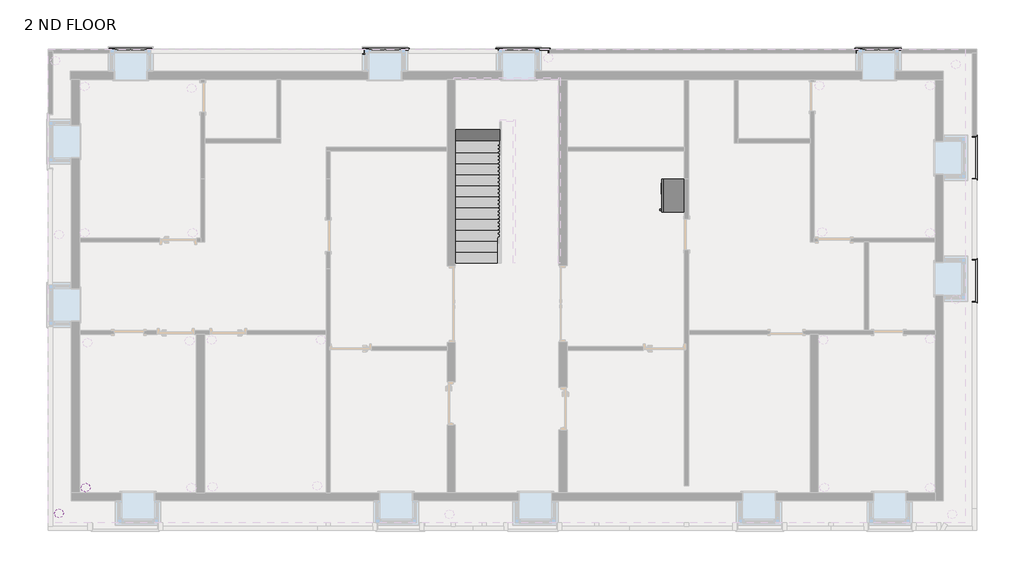
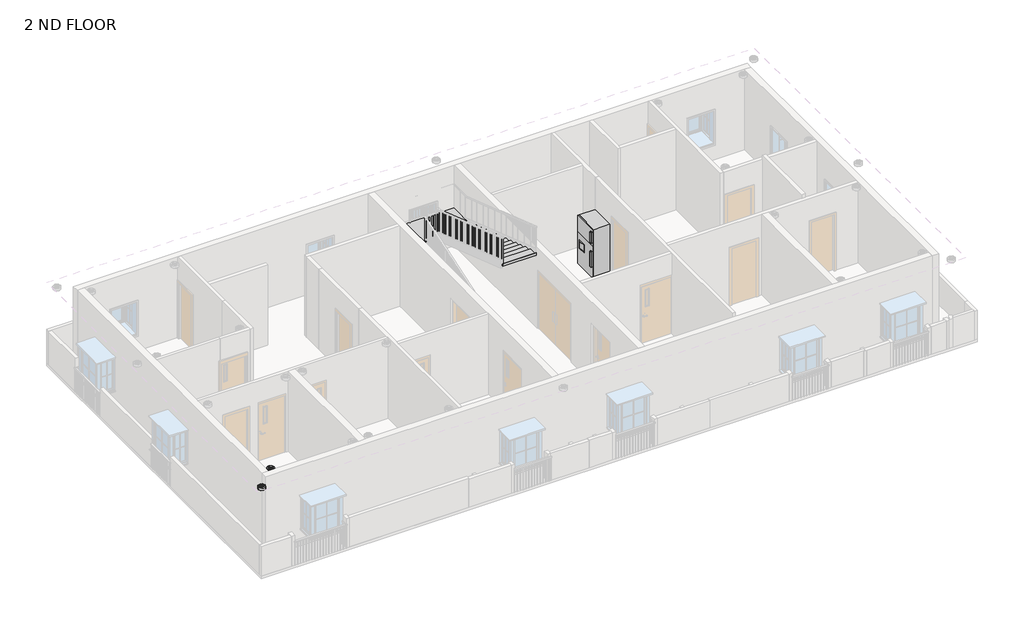
# One storey, part 6 of 7: 6 railings, 2 light fixtures, 1 furniture element, 1 stair flight.
"""IFC4 building model written with IfcOpenShell, lengths in millimetres."""

from ifc_helpers import new_model, si_unit, frame, origin, place, context, project, spatial, polyline, outline, extrude, faceted_brep, transform, mapped, element, save
from components import furniture_65fa61b5, ceiling_light_flat_round_60w_120v_7c4c2a52, stair_flight_d167e677

model = new_model("IFC4")

# Units and contexts
model_context = context("Model", 3, world=origin())
ifc_project = project(units=[si_unit("LENGTHUNIT", "METRE", prefix="MILLI")], contexts=[model_context])

# Site, building, storey
site = spatial("IfcSite", under=ifc_project)
building = spatial("IfcBuilding", under=site)
storey = spatial("IfcBuildingStorey", under=building, Name="2 ND FLOOR", Elevation=6400.8)

# Furniture
placement = place(None, origin())
furniture_shape = furniture_65fa61b5(model_context)
element("IfcFurniture", 1, at=placement, inside=storey, context=model_context, shape_type="MappedRepresentation", body=[
    mapped(furniture_shape, transform((4507.551208, 3815.4567334, 6400.8), x_axis=(0.0, -1.0, 0.0), y_axis=(1.0, 0.0, 0.0), z_axis=(0.0, 0.0, 1.0))),
])

# Light fixtures
ceiling_light_flat_round_60w_120v_shape = ceiling_light_flat_round_60w_120v_7c4c2a52(model_context)
element("IfcLightFixture", 2, ObjectType="Ceiling Light - Flat Round : 60W - 120V", at=placement, inside=storey, context=model_context, shape_type="MappedRepresentation", body=[
    mapped(ceiling_light_flat_round_60w_120v_shape, transform((-12796.1987925, -4356.9932193, 7010.4), x_axis=(1.0, 0.0, 0.0), y_axis=(0.0, 1.0, 0.0), z_axis=(0.0, 0.0, 1.0))),
])
element("IfcLightFixture", 3, ObjectType="Ceiling Light - Flat Round : 60W - 120V", at=placement, inside=storey, context=model_context, shape_type="MappedRepresentation", body=[
    mapped(ceiling_light_flat_round_60w_120v_shape, transform((-12059.5987925, -3645.7932193, 7010.4), x_axis=(1.0, 0.0, 0.0), y_axis=(0.0, 1.0, 0.0), z_axis=(0.0, 0.0, 1.0))),
])

# Railings
element("IfcRailing", 4, ObjectType="Handrail - Rectangular", at=placement, inside=storey, context=model_context, shape_type="SolidModel", body=[
    faceted_brep([(-11412.4067989, 8355.7067329, 7315.2), (-11412.4067989, 8355.7067329, 7264.4), (-11361.6067989, 8355.7067329, 7264.4), (-11361.6067989, 8355.7067329, 7315.2), (-11412.4067989, 8495.4067329, 7315.2), (-11412.4067989, 8495.4067329, 7264.4), (-11361.6067989, 8444.6067329, 7264.4), (-11361.6067989, 8444.6067329, 7315.2), (-10231.3067989, 8495.4067329, 7315.2), (-10231.3067989, 8495.4067329, 7264.4), (-10282.1067989, 8444.6067329, 7264.4), (-10282.1067989, 8444.6067329, 7315.2), (-10231.3067989, 8368.4067329, 7315.2), (-10282.1067989, 8368.4067329, 7315.2), (-10282.1067989, 8368.4067329, 7264.4), (-10231.3067989, 8368.4067329, 7264.4)], [[[0, 1, 2, 3]], [[1, 0, 4, 5]], [[2, 1, 5, 6]], [[3, 2, 6, 7]], [[0, 3, 7, 4]], [[5, 4, 8, 9]], [[6, 5, 9, 10]], [[7, 6, 10, 11]], [[4, 7, 11, 8]], [[12, 13, 14, 15]], [[9, 8, 12, 15]], [[10, 9, 15, 14]], [[11, 10, 14, 13]], [[8, 11, 13, 12]]]),
    extrude(outline(polyline([(-10278.9317989, 8460.4817329), (-10278.9317989, 8479.5317329), (-10259.8817989, 8479.5317329), (-10259.8817989, 8460.4817329), (-10278.9317989, 8460.4817329)])), frame((0.0, 0.0, 6400.8), z_axis=(0.0, 0.0, 1.0), x_axis=(1.0, 0.0, 0.0)), (0.0, 0.0, 1.0), 863.6),
    extrude(outline(polyline([(-10380.5317989, 8460.4817329), (-10380.5317989, 8479.5317329), (-10361.4817989, 8479.5317329), (-10361.4817989, 8460.4817329), (-10380.5317989, 8460.4817329)])), frame((0.0, 0.0, 6400.8), z_axis=(0.0, 0.0, 1.0), x_axis=(1.0, 0.0, 0.0)), (0.0, 0.0, 1.0), 863.6),
    extrude(outline(polyline([(-10482.1317989, 8460.4817329), (-10482.1317989, 8479.5317329), (-10463.0817989, 8479.5317329), (-10463.0817989, 8460.4817329), (-10482.1317989, 8460.4817329)])), frame((0.0, 0.0, 6400.8), z_axis=(0.0, 0.0, 1.0), x_axis=(1.0, 0.0, 0.0)), (0.0, 0.0, 1.0), 863.6),
    extrude(outline(polyline([(-10583.7317989, 8460.4817329), (-10583.7317989, 8479.5317329), (-10564.6817989, 8479.5317329), (-10564.6817989, 8460.4817329), (-10583.7317989, 8460.4817329)])), frame((0.0, 0.0, 6400.8), z_axis=(0.0, 0.0, 1.0), x_axis=(1.0, 0.0, 0.0)), (0.0, 0.0, 1.0), 863.6),
    extrude(outline(polyline([(-10685.3317989, 8460.4817329), (-10685.3317989, 8479.5317329), (-10666.2817989, 8479.5317329), (-10666.2817989, 8460.4817329), (-10685.3317989, 8460.4817329)])), frame((0.0, 0.0, 6400.8), z_axis=(0.0, 0.0, 1.0), x_axis=(1.0, 0.0, 0.0)), (0.0, 0.0, 1.0), 863.6),
    extrude(outline(polyline([(-10786.9317989, 8460.4817329), (-10786.9317989, 8479.5317329), (-10767.8817989, 8479.5317329), (-10767.8817989, 8460.4817329), (-10786.9317989, 8460.4817329)])), frame((0.0, 0.0, 6400.8), z_axis=(0.0, 0.0, 1.0), x_axis=(1.0, 0.0, 0.0)), (0.0, 0.0, 1.0), 863.6),
    extrude(outline(polyline([(-10888.5317989, 8460.4817329), (-10888.5317989, 8479.5317329), (-10869.4817989, 8479.5317329), (-10869.4817989, 8460.4817329), (-10888.5317989, 8460.4817329)])), frame((0.0, 0.0, 6400.8), z_axis=(0.0, 0.0, 1.0), x_axis=(1.0, 0.0, 0.0)), (0.0, 0.0, 1.0), 863.6),
    extrude(outline(polyline([(-10990.1317989, 8460.4817329), (-10990.1317989, 8479.5317329), (-10971.0817989, 8479.5317329), (-10971.0817989, 8460.4817329), (-10990.1317989, 8460.4817329)])), frame((0.0, 0.0, 6400.8), z_axis=(0.0, 0.0, 1.0), x_axis=(1.0, 0.0, 0.0)), (0.0, 0.0, 1.0), 863.6),
    extrude(outline(polyline([(-11091.7317989, 8460.4817329), (-11091.7317989, 8479.5317329), (-11072.6817989, 8479.5317329), (-11072.6817989, 8460.4817329), (-11091.7317989, 8460.4817329)])), frame((0.0, 0.0, 6400.8), z_axis=(0.0, 0.0, 1.0), x_axis=(1.0, 0.0, 0.0)), (0.0, 0.0, 1.0), 863.6),
    extrude(outline(polyline([(-11193.3317989, 8460.4817329), (-11193.3317989, 8479.5317329), (-11174.2817989, 8479.5317329), (-11174.2817989, 8460.4817329), (-11193.3317989, 8460.4817329)])), frame((0.0, 0.0, 6400.8), z_axis=(0.0, 0.0, 1.0), x_axis=(1.0, 0.0, 0.0)), (0.0, 0.0, 1.0), 863.6),
    extrude(outline(polyline([(-11294.9317989, 8460.4817329), (-11294.9317989, 8479.5317329), (-11275.8817989, 8479.5317329), (-11275.8817989, 8460.4817329), (-11294.9317989, 8460.4817329)])), frame((0.0, 0.0, 6400.8), z_axis=(0.0, 0.0, 1.0), x_axis=(1.0, 0.0, 0.0)), (0.0, 0.0, 1.0), 863.6),
    extrude(outline(polyline([(-11377.4817989, 8447.7817329), (-11396.5317989, 8447.7817329), (-11396.5317989, 8466.8317329), (-11377.4817989, 8466.8317329), (-11377.4817989, 8447.7817329)])), frame((0.0, 0.0, 6400.8), z_axis=(0.0, 0.0, 1.0), x_axis=(1.0, 0.0, 0.0)), (0.0, 0.0, 1.0), 863.6),
    extrude(outline(polyline([(-10266.2317989, 8460.4817329), (-10266.2317989, 8479.5317329), (-10247.1817989, 8479.5317329), (-10247.1817989, 8460.4817329), (-10266.2317989, 8460.4817329)])), frame((0.0, 0.0, 6400.8), z_axis=(0.0, 0.0, 1.0), x_axis=(1.0, 0.0, 0.0)), (0.0, 0.0, 1.0), 863.6),
    extrude(outline(polyline([(-11377.4817989, 8460.4817329), (-11396.5317989, 8460.4817329), (-11396.5317989, 8479.5317329), (-11377.4817989, 8479.5317329), (-11377.4817989, 8460.4817329)])), frame((0.0, 0.0, 6400.8), z_axis=(0.0, 0.0, 1.0), x_axis=(1.0, 0.0, 0.0)), (0.0, 0.0, 1.0), 863.6),
    extrude(outline(polyline([(-10266.2317989, 8387.4567329), (-10247.1817989, 8387.4567329), (-10247.1817989, 8368.4067329), (-10266.2317989, 8368.4067329), (-10266.2317989, 8387.4567329)])), frame((0.0, 0.0, 6400.8), z_axis=(0.0, 0.0, 1.0), x_axis=(1.0, 0.0, 0.0)), (0.0, 0.0, 1.0), 863.6),
    extrude(outline(polyline([(-11377.4817989, 8355.7067329), (-11396.5317989, 8355.7067329), (-11396.5317989, 8374.7567329), (-11377.4817989, 8374.7567329), (-11377.4817989, 8355.7067329)])), frame((0.0, 0.0, 6400.8), z_axis=(0.0, 0.0, 1.0), x_axis=(1.0, 0.0, 0.0)), (0.0, 0.0, 1.0), 863.6),
])
element("IfcRailing", 5, ObjectType="Handrail - Rectangular", at=placement, inside=storey, context=model_context, shape_type="SolidModel", body=[
    faceted_brep([(-4407.8487992, 8336.6567329, 7315.2), (-4407.8487992, 8336.6567329, 7264.4), (-4357.0487992, 8336.6567329, 7264.4), (-4357.0487992, 8336.6567329, 7315.2), (-4407.8487992, 8495.4067329, 7315.2), (-4407.8487992, 8495.4067329, 7264.4), (-4357.0487992, 8444.6067329, 7264.4), (-4357.0487992, 8444.6067329, 7315.2), (-3120.4490672, 8495.4067329, 7315.2), (-3120.4490672, 8444.6067329, 7315.2), (-3120.4490672, 8444.6067329, 7264.4), (-3120.4490672, 8495.4067329, 7264.4)], [[[0, 1, 2, 3]], [[1, 0, 4, 5]], [[2, 1, 5, 6]], [[3, 2, 6, 7]], [[0, 3, 7, 4]], [[8, 9, 10, 11]], [[5, 4, 8, 11]], [[6, 5, 11, 10]], [[7, 6, 10, 9]], [[4, 7, 9, 8]]]),
    extrude(outline(polyline([(-3172.7737992, 8460.4817329), (-3172.7737992, 8479.5317329), (-3153.7237992, 8479.5317329), (-3153.7237992, 8460.4817329), (-3172.7737992, 8460.4817329)])), frame((0.0, 0.0, 6400.8), z_axis=(0.0, 0.0, 1.0), x_axis=(1.0, 0.0, 0.0)), (0.0, 0.0, 1.0), 863.6),
    extrude(outline(polyline([(-3274.3737992, 8460.4817329), (-3274.3737992, 8479.5317329), (-3255.3237992, 8479.5317329), (-3255.3237992, 8460.4817329), (-3274.3737992, 8460.4817329)])), frame((0.0, 0.0, 6400.8), z_axis=(0.0, 0.0, 1.0), x_axis=(1.0, 0.0, 0.0)), (0.0, 0.0, 1.0), 863.6),
    extrude(outline(polyline([(-3375.9737992, 8460.4817329), (-3375.9737992, 8479.5317329), (-3356.9237992, 8479.5317329), (-3356.9237992, 8460.4817329), (-3375.9737992, 8460.4817329)])), frame((0.0, 0.0, 6400.8), z_axis=(0.0, 0.0, 1.0), x_axis=(1.0, 0.0, 0.0)), (0.0, 0.0, 1.0), 863.6),
    extrude(outline(polyline([(-3477.5737992, 8460.4817329), (-3477.5737992, 8479.5317329), (-3458.5237992, 8479.5317329), (-3458.5237992, 8460.4817329), (-3477.5737992, 8460.4817329)])), frame((0.0, 0.0, 6400.8), z_axis=(0.0, 0.0, 1.0), x_axis=(1.0, 0.0, 0.0)), (0.0, 0.0, 1.0), 863.6),
    extrude(outline(polyline([(-3579.1737992, 8460.4817329), (-3579.1737992, 8479.5317329), (-3560.1237992, 8479.5317329), (-3560.1237992, 8460.4817329), (-3579.1737992, 8460.4817329)])), frame((0.0, 0.0, 6400.8), z_axis=(0.0, 0.0, 1.0), x_axis=(1.0, 0.0, 0.0)), (0.0, 0.0, 1.0), 863.6),
    extrude(outline(polyline([(-3680.7737992, 8460.4817329), (-3680.7737992, 8479.5317329), (-3661.7237992, 8479.5317329), (-3661.7237992, 8460.4817329), (-3680.7737992, 8460.4817329)])), frame((0.0, 0.0, 6400.8), z_axis=(0.0, 0.0, 1.0), x_axis=(1.0, 0.0, 0.0)), (0.0, 0.0, 1.0), 863.6),
    extrude(outline(polyline([(-3782.3737992, 8460.4817329), (-3782.3737992, 8479.5317329), (-3763.3237992, 8479.5317329), (-3763.3237992, 8460.4817329), (-3782.3737992, 8460.4817329)])), frame((0.0, 0.0, 6400.8), z_axis=(0.0, 0.0, 1.0), x_axis=(1.0, 0.0, 0.0)), (0.0, 0.0, 1.0), 863.6),
    extrude(outline(polyline([(-3883.9737992, 8460.4817329), (-3883.9737992, 8479.5317329), (-3864.9237992, 8479.5317329), (-3864.9237992, 8460.4817329), (-3883.9737992, 8460.4817329)])), frame((0.0, 0.0, 6400.8), z_axis=(0.0, 0.0, 1.0), x_axis=(1.0, 0.0, 0.0)), (0.0, 0.0, 1.0), 863.6),
    extrude(outline(polyline([(-3985.5737992, 8460.4817329), (-3985.5737992, 8479.5317329), (-3966.5237992, 8479.5317329), (-3966.5237992, 8460.4817329), (-3985.5737992, 8460.4817329)])), frame((0.0, 0.0, 6400.8), z_axis=(0.0, 0.0, 1.0), x_axis=(1.0, 0.0, 0.0)), (0.0, 0.0, 1.0), 863.6),
    extrude(outline(polyline([(-4087.1737992, 8460.4817329), (-4087.1737992, 8479.5317329), (-4068.1237992, 8479.5317329), (-4068.1237992, 8460.4817329), (-4087.1737992, 8460.4817329)])), frame((0.0, 0.0, 6400.8), z_axis=(0.0, 0.0, 1.0), x_axis=(1.0, 0.0, 0.0)), (0.0, 0.0, 1.0), 863.6),
    extrude(outline(polyline([(-4188.7737992, 8460.4817329), (-4188.7737992, 8479.5317329), (-4169.7237992, 8479.5317329), (-4169.7237992, 8460.4817329), (-4188.7737992, 8460.4817329)])), frame((0.0, 0.0, 6400.8), z_axis=(0.0, 0.0, 1.0), x_axis=(1.0, 0.0, 0.0)), (0.0, 0.0, 1.0), 863.6),
    extrude(outline(polyline([(-4290.3737992, 8460.4817329), (-4290.3737992, 8479.5317329), (-4271.3237992, 8479.5317329), (-4271.3237992, 8460.4817329), (-4290.3737992, 8460.4817329)])), frame((0.0, 0.0, 6400.8), z_axis=(0.0, 0.0, 1.0), x_axis=(1.0, 0.0, 0.0)), (0.0, 0.0, 1.0), 863.6),
    extrude(outline(polyline([(-4372.9237992, 8428.7317329), (-4391.9737992, 8428.7317329), (-4391.9737992, 8447.7817329), (-4372.9237992, 8447.7817329), (-4372.9237992, 8428.7317329)])), frame((0.0, 0.0, 6400.8), z_axis=(0.0, 0.0, 1.0), x_axis=(1.0, 0.0, 0.0)), (0.0, 0.0, 1.0), 863.6),
    extrude(outline(polyline([(-4372.9237992, 8460.4817329), (-4391.9737992, 8460.4817329), (-4391.9737992, 8479.5317329), (-4372.9237992, 8479.5317329), (-4372.9237992, 8460.4817329)])), frame((0.0, 0.0, 6400.8), z_axis=(0.0, 0.0, 1.0), x_axis=(1.0, 0.0, 0.0)), (0.0, 0.0, 1.0), 863.6),
    extrude(outline(polyline([(-3139.4990672, 8460.4817329), (-3139.4990672, 8479.5317329), (-3120.4490672, 8479.5317329), (-3120.4490672, 8460.4817329), (-3139.4990672, 8460.4817329)])), frame((0.0, 0.0, 6400.8), z_axis=(0.0, 0.0, 1.0), x_axis=(1.0, 0.0, 0.0)), (0.0, 0.0, 1.0), 863.6),
    extrude(outline(polyline([(-4372.9237992, 8336.6567329), (-4391.9737992, 8336.6567329), (-4391.9737992, 8355.7067329), (-4372.9237992, 8355.7067329), (-4372.9237992, 8336.6567329)])), frame((0.0, 0.0, 6400.8), z_axis=(0.0, 0.0, 1.0), x_axis=(1.0, 0.0, 0.0)), (0.0, 0.0, 1.0), 863.6),
])
element("IfcRailing", 6, ObjectType="Handrail - Rectangular", at=placement, inside=storey, context=model_context, shape_type="SolidModel", body=[
    faceted_brep([(-732.8490672, 8355.7067329, 7315.2), (-732.8490672, 8355.7067329, 7264.4), (-682.0490672, 8355.7067329, 7264.4), (-682.0490672, 8355.7067329, 7315.2), (-732.8490672, 8495.4067329, 7315.2), (-732.8490672, 8495.4067329, 7264.4), (-682.0490672, 8444.6067329, 7264.4), (-682.0490672, 8444.6067329, 7315.2), (766.8932011, 8495.4067329, 7315.2), (766.8932011, 8495.4067329, 7264.4), (716.0932011, 8444.6067329, 7264.4), (716.0932011, 8444.6067329, 7315.2), (766.8932011, 8355.7067329, 7315.2), (716.0932011, 8355.7067329, 7315.2), (716.0932011, 8355.7067329, 7264.4), (766.8932011, 8355.7067329, 7264.4)], [[[0, 1, 2, 3]], [[1, 0, 4, 5]], [[2, 1, 5, 6]], [[3, 2, 6, 7]], [[0, 3, 7, 4]], [[5, 4, 8, 9]], [[6, 5, 9, 10]], [[7, 6, 10, 11]], [[4, 7, 11, 8]], [[12, 13, 14, 15]], [[9, 8, 12, 15]], [[10, 9, 15, 14]], [[11, 10, 14, 13]], [[8, 11, 13, 12]]]),
    extrude(outline(polyline([(731.9682011, 8377.9317329), (751.0182011, 8377.9317329), (751.0182011, 8358.8817329), (731.9682011, 8358.8817329), (731.9682011, 8377.9317329)])), frame((0.0, 0.0, 6400.8), z_axis=(0.0, 0.0, 1.0), x_axis=(1.0, 0.0, 0.0)), (0.0, 0.0, 1.0), 863.6),
    extrude(outline(polyline([(705.4259328, 8460.4817329), (705.4259328, 8479.5317329), (724.4759328, 8479.5317329), (724.4759328, 8460.4817329), (705.4259328, 8460.4817329)])), frame((0.0, 0.0, 6400.8), z_axis=(0.0, 0.0, 1.0), x_axis=(1.0, 0.0, 0.0)), (0.0, 0.0, 1.0), 863.6),
    extrude(outline(polyline([(603.8259328, 8460.4817329), (603.8259328, 8479.5317329), (622.8759328, 8479.5317329), (622.8759328, 8460.4817329), (603.8259328, 8460.4817329)])), frame((0.0, 0.0, 6400.8), z_axis=(0.0, 0.0, 1.0), x_axis=(1.0, 0.0, 0.0)), (0.0, 0.0, 1.0), 863.6),
    extrude(outline(polyline([(502.2259328, 8460.4817329), (502.2259328, 8479.5317329), (521.2759328, 8479.5317329), (521.2759328, 8460.4817329), (502.2259328, 8460.4817329)])), frame((0.0, 0.0, 6400.8), z_axis=(0.0, 0.0, 1.0), x_axis=(1.0, 0.0, 0.0)), (0.0, 0.0, 1.0), 863.6),
    extrude(outline(polyline([(400.6259328, 8460.4817329), (400.6259328, 8479.5317329), (419.6759328, 8479.5317329), (419.6759328, 8460.4817329), (400.6259328, 8460.4817329)])), frame((0.0, 0.0, 6400.8), z_axis=(0.0, 0.0, 1.0), x_axis=(1.0, 0.0, 0.0)), (0.0, 0.0, 1.0), 863.6),
    extrude(outline(polyline([(299.0259328, 8460.4817329), (299.0259328, 8479.5317329), (318.0759328, 8479.5317329), (318.0759328, 8460.4817329), (299.0259328, 8460.4817329)])), frame((0.0, 0.0, 6400.8), z_axis=(0.0, 0.0, 1.0), x_axis=(1.0, 0.0, 0.0)), (0.0, 0.0, 1.0), 863.6),
    extrude(outline(polyline([(197.4259328, 8460.4817329), (197.4259328, 8479.5317329), (216.4759328, 8479.5317329), (216.4759328, 8460.4817329), (197.4259328, 8460.4817329)])), frame((0.0, 0.0, 6400.8), z_axis=(0.0, 0.0, 1.0), x_axis=(1.0, 0.0, 0.0)), (0.0, 0.0, 1.0), 863.6),
    extrude(outline(polyline([(95.8259328, 8460.4817329), (95.8259328, 8479.5317329), (114.8759328, 8479.5317329), (114.8759328, 8460.4817329), (95.8259328, 8460.4817329)])), frame((0.0, 0.0, 6400.8), z_axis=(0.0, 0.0, 1.0), x_axis=(1.0, 0.0, 0.0)), (0.0, 0.0, 1.0), 863.6),
    extrude(outline(polyline([(-5.7740672, 8460.4817329), (-5.7740672, 8479.5317329), (13.2759328, 8479.5317329), (13.2759328, 8460.4817329), (-5.7740672, 8460.4817329)])), frame((0.0, 0.0, 6400.8), z_axis=(0.0, 0.0, 1.0), x_axis=(1.0, 0.0, 0.0)), (0.0, 0.0, 1.0), 863.6),
    extrude(outline(polyline([(-107.3740672, 8460.4817329), (-107.3740672, 8479.5317329), (-88.3240672, 8479.5317329), (-88.3240672, 8460.4817329), (-107.3740672, 8460.4817329)])), frame((0.0, 0.0, 6400.8), z_axis=(0.0, 0.0, 1.0), x_axis=(1.0, 0.0, 0.0)), (0.0, 0.0, 1.0), 863.6),
    extrude(outline(polyline([(-208.9740672, 8460.4817329), (-208.9740672, 8479.5317329), (-189.9240672, 8479.5317329), (-189.9240672, 8460.4817329), (-208.9740672, 8460.4817329)])), frame((0.0, 0.0, 6400.8), z_axis=(0.0, 0.0, 1.0), x_axis=(1.0, 0.0, 0.0)), (0.0, 0.0, 1.0), 863.6),
    extrude(outline(polyline([(-310.5740672, 8460.4817329), (-310.5740672, 8479.5317329), (-291.5240672, 8479.5317329), (-291.5240672, 8460.4817329), (-310.5740672, 8460.4817329)])), frame((0.0, 0.0, 6400.8), z_axis=(0.0, 0.0, 1.0), x_axis=(1.0, 0.0, 0.0)), (0.0, 0.0, 1.0), 863.6),
    extrude(outline(polyline([(-412.1740672, 8460.4817329), (-412.1740672, 8479.5317329), (-393.1240672, 8479.5317329), (-393.1240672, 8460.4817329), (-412.1740672, 8460.4817329)])), frame((0.0, 0.0, 6400.8), z_axis=(0.0, 0.0, 1.0), x_axis=(1.0, 0.0, 0.0)), (0.0, 0.0, 1.0), 863.6),
    extrude(outline(polyline([(-513.7740672, 8460.4817329), (-513.7740672, 8479.5317329), (-494.7240672, 8479.5317329), (-494.7240672, 8460.4817329), (-513.7740672, 8460.4817329)])), frame((0.0, 0.0, 6400.8), z_axis=(0.0, 0.0, 1.0), x_axis=(1.0, 0.0, 0.0)), (0.0, 0.0, 1.0), 863.6),
    extrude(outline(polyline([(-615.3740672, 8460.4817329), (-615.3740672, 8479.5317329), (-596.3240672, 8479.5317329), (-596.3240672, 8460.4817329), (-615.3740672, 8460.4817329)])), frame((0.0, 0.0, 6400.8), z_axis=(0.0, 0.0, 1.0), x_axis=(1.0, 0.0, 0.0)), (0.0, 0.0, 1.0), 863.6),
    extrude(outline(polyline([(-697.9240672, 8447.7817329), (-716.9740672, 8447.7817329), (-716.9740672, 8466.8317329), (-697.9240672, 8466.8317329), (-697.9240672, 8447.7817329)])), frame((0.0, 0.0, 6400.8), z_axis=(0.0, 0.0, 1.0), x_axis=(1.0, 0.0, 0.0)), (0.0, 0.0, 1.0), 863.6),
    extrude(outline(polyline([(731.9682011, 8460.4817329), (731.9682011, 8479.5317329), (751.0182011, 8479.5317329), (751.0182011, 8460.4817329), (731.9682011, 8460.4817329)])), frame((0.0, 0.0, 6400.8), z_axis=(0.0, 0.0, 1.0), x_axis=(1.0, 0.0, 0.0)), (0.0, 0.0, 1.0), 863.6),
    extrude(outline(polyline([(-697.9240672, 8460.4817329), (-716.9740672, 8460.4817329), (-716.9740672, 8479.5317329), (-697.9240672, 8479.5317329), (-697.9240672, 8460.4817329)])), frame((0.0, 0.0, 6400.8), z_axis=(0.0, 0.0, 1.0), x_axis=(1.0, 0.0, 0.0)), (0.0, 0.0, 1.0), 863.6),
    extrude(outline(polyline([(731.9682011, 8374.7567329), (751.0182011, 8374.7567329), (751.0182011, 8355.7067329), (731.9682011, 8355.7067329), (731.9682011, 8374.7567329)])), frame((0.0, 0.0, 6400.8), z_axis=(0.0, 0.0, 1.0), x_axis=(1.0, 0.0, 0.0)), (0.0, 0.0, 1.0), 863.6),
    extrude(outline(polyline([(-697.9240672, 8355.7067329), (-716.9740672, 8355.7067329), (-716.9740672, 8374.7567329), (-697.9240672, 8374.7567329), (-697.9240672, 8355.7067329)])), frame((0.0, 0.0, 6400.8), z_axis=(0.0, 0.0, 1.0), x_axis=(1.0, 0.0, 0.0)), (0.0, 0.0, 1.0), 863.6),
])
element("IfcRailing", 7, ObjectType="Handrail - Rectangular", at=placement, inside=storey, context=model_context, shape_type="SolidModel", body=[
    faceted_brep([(9174.2932011, 8355.7067329, 7315.2), (9174.2932011, 8355.7067329, 7264.4), (9225.0932011, 8355.7067329, 7264.4), (9225.0932011, 8355.7067329, 7315.2), (9174.2932011, 8495.4067329, 7315.2), (9174.2932011, 8495.4067329, 7264.4), (9225.0932011, 8444.6067329, 7264.4), (9225.0932011, 8444.6067329, 7315.2), (10462.2009401, 8495.4067329, 7315.2), (10462.2009401, 8444.6067329, 7315.2), (10462.2009401, 8444.6067329, 7264.4), (10462.2009401, 8495.4067329, 7264.4)], [[[0, 1, 2, 3]], [[1, 0, 4, 5]], [[2, 1, 5, 6]], [[3, 2, 6, 7]], [[0, 3, 7, 4]], [[8, 9, 10, 11]], [[5, 4, 8, 11]], [[6, 5, 11, 10]], [[7, 6, 10, 9]], [[4, 7, 9, 8]]]),
    extrude(outline(polyline([(10409.3682011, 8460.4817329), (10409.3682011, 8479.5317329), (10428.4182011, 8479.5317329), (10428.4182011, 8460.4817329), (10409.3682011, 8460.4817329)])), frame((0.0, 0.0, 6400.8), z_axis=(0.0, 0.0, 1.0), x_axis=(1.0, 0.0, 0.0)), (0.0, 0.0, 1.0), 863.6),
    extrude(outline(polyline([(10307.7682011, 8460.4817329), (10307.7682011, 8479.5317329), (10326.8182011, 8479.5317329), (10326.8182011, 8460.4817329), (10307.7682011, 8460.4817329)])), frame((0.0, 0.0, 6400.8), z_axis=(0.0, 0.0, 1.0), x_axis=(1.0, 0.0, 0.0)), (0.0, 0.0, 1.0), 863.6),
    extrude(outline(polyline([(10206.1682011, 8460.4817329), (10206.1682011, 8479.5317329), (10225.2182011, 8479.5317329), (10225.2182011, 8460.4817329), (10206.1682011, 8460.4817329)])), frame((0.0, 0.0, 6400.8), z_axis=(0.0, 0.0, 1.0), x_axis=(1.0, 0.0, 0.0)), (0.0, 0.0, 1.0), 863.6),
    extrude(outline(polyline([(10104.5682011, 8460.4817329), (10104.5682011, 8479.5317329), (10123.6182011, 8479.5317329), (10123.6182011, 8460.4817329), (10104.5682011, 8460.4817329)])), frame((0.0, 0.0, 6400.8), z_axis=(0.0, 0.0, 1.0), x_axis=(1.0, 0.0, 0.0)), (0.0, 0.0, 1.0), 863.6),
    extrude(outline(polyline([(10002.9682011, 8460.4817329), (10002.9682011, 8479.5317329), (10022.0182011, 8479.5317329), (10022.0182011, 8460.4817329), (10002.9682011, 8460.4817329)])), frame((0.0, 0.0, 6400.8), z_axis=(0.0, 0.0, 1.0), x_axis=(1.0, 0.0, 0.0)), (0.0, 0.0, 1.0), 863.6),
    extrude(outline(polyline([(9901.3682011, 8460.4817329), (9901.3682011, 8479.5317329), (9920.4182011, 8479.5317329), (9920.4182011, 8460.4817329), (9901.3682011, 8460.4817329)])), frame((0.0, 0.0, 6400.8), z_axis=(0.0, 0.0, 1.0), x_axis=(1.0, 0.0, 0.0)), (0.0, 0.0, 1.0), 863.6),
    extrude(outline(polyline([(9799.7682011, 8460.4817329), (9799.7682011, 8479.5317329), (9818.8182011, 8479.5317329), (9818.8182011, 8460.4817329), (9799.7682011, 8460.4817329)])), frame((0.0, 0.0, 6400.8), z_axis=(0.0, 0.0, 1.0), x_axis=(1.0, 0.0, 0.0)), (0.0, 0.0, 1.0), 863.6),
    extrude(outline(polyline([(9698.1682011, 8460.4817329), (9698.1682011, 8479.5317329), (9717.2182011, 8479.5317329), (9717.2182011, 8460.4817329), (9698.1682011, 8460.4817329)])), frame((0.0, 0.0, 6400.8), z_axis=(0.0, 0.0, 1.0), x_axis=(1.0, 0.0, 0.0)), (0.0, 0.0, 1.0), 863.6),
    extrude(outline(polyline([(9596.5682011, 8460.4817329), (9596.5682011, 8479.5317329), (9615.6182011, 8479.5317329), (9615.6182011, 8460.4817329), (9596.5682011, 8460.4817329)])), frame((0.0, 0.0, 6400.8), z_axis=(0.0, 0.0, 1.0), x_axis=(1.0, 0.0, 0.0)), (0.0, 0.0, 1.0), 863.6),
    extrude(outline(polyline([(9494.9682011, 8460.4817329), (9494.9682011, 8479.5317329), (9514.0182011, 8479.5317329), (9514.0182011, 8460.4817329), (9494.9682011, 8460.4817329)])), frame((0.0, 0.0, 6400.8), z_axis=(0.0, 0.0, 1.0), x_axis=(1.0, 0.0, 0.0)), (0.0, 0.0, 1.0), 863.6),
    extrude(outline(polyline([(9393.3682011, 8460.4817329), (9393.3682011, 8479.5317329), (9412.4182011, 8479.5317329), (9412.4182011, 8460.4817329), (9393.3682011, 8460.4817329)])), frame((0.0, 0.0, 6400.8), z_axis=(0.0, 0.0, 1.0), x_axis=(1.0, 0.0, 0.0)), (0.0, 0.0, 1.0), 863.6),
    extrude(outline(polyline([(9291.7682011, 8460.4817329), (9291.7682011, 8479.5317329), (9310.8182011, 8479.5317329), (9310.8182011, 8460.4817329), (9291.7682011, 8460.4817329)])), frame((0.0, 0.0, 6400.8), z_axis=(0.0, 0.0, 1.0), x_axis=(1.0, 0.0, 0.0)), (0.0, 0.0, 1.0), 863.6),
    extrude(outline(polyline([(9209.2182011, 8447.7817329), (9190.1682011, 8447.7817329), (9190.1682011, 8466.8317329), (9209.2182011, 8466.8317329), (9209.2182011, 8447.7817329)])), frame((0.0, 0.0, 6400.8), z_axis=(0.0, 0.0, 1.0), x_axis=(1.0, 0.0, 0.0)), (0.0, 0.0, 1.0), 863.6),
    extrude(outline(polyline([(9209.2182011, 8460.4817329), (9190.1682011, 8460.4817329), (9190.1682011, 8479.5317329), (9209.2182011, 8479.5317329), (9209.2182011, 8460.4817329)])), frame((0.0, 0.0, 6400.8), z_axis=(0.0, 0.0, 1.0), x_axis=(1.0, 0.0, 0.0)), (0.0, 0.0, 1.0), 863.6),
    extrude(outline(polyline([(10443.1509401, 8460.4817329), (10443.1509401, 8479.5317329), (10462.2009401, 8479.5317329), (10462.2009401, 8460.4817329), (10443.1509401, 8460.4817329)])), frame((0.0, 0.0, 6400.8), z_axis=(0.0, 0.0, 1.0), x_axis=(1.0, 0.0, 0.0)), (0.0, 0.0, 1.0), 863.6),
    extrude(outline(polyline([(9209.2182011, 8355.7067329), (9190.1682011, 8355.7067329), (9190.1682011, 8374.7567329), (9209.2182011, 8374.7567329), (9209.2182011, 8355.7067329)])), frame((0.0, 0.0, 6400.8), z_axis=(0.0, 0.0, 1.0), x_axis=(1.0, 0.0, 0.0)), (0.0, 0.0, 1.0), 863.6),
])
element("IfcRailing", 8, ObjectType="Handrail - Rectangular", at=placement, inside=storey, context=model_context, shape_type="SolidModel", body=[
    faceted_brep([(12426.0012043, 2691.5067329, 7315.2), (12426.0012043, 2691.5067329, 7264.4), (12426.0012043, 2640.7067329, 7264.4), (12426.0012043, 2640.7067329, 7315.2), (12565.7012043, 2691.5067329, 7315.2), (12565.7012043, 2691.5067329, 7264.4), (12514.9012043, 2640.7067329, 7264.4), (12514.9012043, 2640.7067329, 7315.2), (12565.7012043, 1453.2567334, 7315.2), (12565.7012043, 1453.2567334, 7264.4), (12514.9012043, 1504.0567334, 7264.4), (12514.9012043, 1504.0567334, 7315.2), (12426.0012043, 1453.2567334, 7315.2), (12426.0012043, 1504.0567334, 7315.2), (12426.0012043, 1504.0567334, 7264.4), (12426.0012043, 1453.2567334, 7264.4)], [[[0, 1, 2, 3]], [[1, 0, 4, 5]], [[2, 1, 5, 6]], [[3, 2, 6, 7]], [[0, 3, 7, 4]], [[5, 4, 8, 9]], [[6, 5, 9, 10]], [[7, 6, 10, 11]], [[4, 7, 11, 8]], [[12, 13, 14, 15]], [[9, 8, 12, 15]], [[10, 9, 15, 14]], [[11, 10, 14, 13]], [[8, 11, 13, 12]]]),
    extrude(outline(polyline([(12448.2262043, 1488.1817334), (12448.2262043, 1469.1317334), (12429.1762043, 1469.1317334), (12429.1762043, 1488.1817334), (12448.2262043, 1488.1817334)])), frame((0.0, 0.0, 6400.8), z_axis=(0.0, 0.0, 1.0), x_axis=(1.0, 0.0, 0.0)), (0.0, 0.0, 1.0), 863.6),
    extrude(outline(polyline([(12530.7762043, 1558.0317329), (12549.8262043, 1558.0317329), (12549.8262043, 1538.9817329), (12530.7762043, 1538.9817329), (12530.7762043, 1558.0317329)])), frame((0.0, 0.0, 6400.8), z_axis=(0.0, 0.0, 1.0), x_axis=(1.0, 0.0, 0.0)), (0.0, 0.0, 1.0), 863.6),
    extrude(outline(polyline([(12530.7762043, 1659.6317329), (12549.8262043, 1659.6317329), (12549.8262043, 1640.5817329), (12530.7762043, 1640.5817329), (12530.7762043, 1659.6317329)])), frame((0.0, 0.0, 6400.8), z_axis=(0.0, 0.0, 1.0), x_axis=(1.0, 0.0, 0.0)), (0.0, 0.0, 1.0), 863.6),
    extrude(outline(polyline([(12530.7762043, 1761.2317329), (12549.8262043, 1761.2317329), (12549.8262043, 1742.1817329), (12530.7762043, 1742.1817329), (12530.7762043, 1761.2317329)])), frame((0.0, 0.0, 6400.8), z_axis=(0.0, 0.0, 1.0), x_axis=(1.0, 0.0, 0.0)), (0.0, 0.0, 1.0), 863.6),
    extrude(outline(polyline([(12530.7762043, 1862.8317329), (12549.8262043, 1862.8317329), (12549.8262043, 1843.7817329), (12530.7762043, 1843.7817329), (12530.7762043, 1862.8317329)])), frame((0.0, 0.0, 6400.8), z_axis=(0.0, 0.0, 1.0), x_axis=(1.0, 0.0, 0.0)), (0.0, 0.0, 1.0), 863.6),
    extrude(outline(polyline([(12530.7762043, 1964.4317329), (12549.8262043, 1964.4317329), (12549.8262043, 1945.3817329), (12530.7762043, 1945.3817329), (12530.7762043, 1964.4317329)])), frame((0.0, 0.0, 6400.8), z_axis=(0.0, 0.0, 1.0), x_axis=(1.0, 0.0, 0.0)), (0.0, 0.0, 1.0), 863.6),
    extrude(outline(polyline([(12530.7762043, 2066.0317329), (12549.8262043, 2066.0317329), (12549.8262043, 2046.9817329), (12530.7762043, 2046.9817329), (12530.7762043, 2066.0317329)])), frame((0.0, 0.0, 6400.8), z_axis=(0.0, 0.0, 1.0), x_axis=(1.0, 0.0, 0.0)), (0.0, 0.0, 1.0), 863.6),
    extrude(outline(polyline([(12530.7762043, 2167.6317329), (12549.8262043, 2167.6317329), (12549.8262043, 2148.5817329), (12530.7762043, 2148.5817329), (12530.7762043, 2167.6317329)])), frame((0.0, 0.0, 6400.8), z_axis=(0.0, 0.0, 1.0), x_axis=(1.0, 0.0, 0.0)), (0.0, 0.0, 1.0), 863.6),
    extrude(outline(polyline([(12530.7762043, 2269.2317329), (12549.8262043, 2269.2317329), (12549.8262043, 2250.1817329), (12530.7762043, 2250.1817329), (12530.7762043, 2269.2317329)])), frame((0.0, 0.0, 6400.8), z_axis=(0.0, 0.0, 1.0), x_axis=(1.0, 0.0, 0.0)), (0.0, 0.0, 1.0), 863.6),
    extrude(outline(polyline([(12530.7762043, 2370.8317329), (12549.8262043, 2370.8317329), (12549.8262043, 2351.7817329), (12530.7762043, 2351.7817329), (12530.7762043, 2370.8317329)])), frame((0.0, 0.0, 6400.8), z_axis=(0.0, 0.0, 1.0), x_axis=(1.0, 0.0, 0.0)), (0.0, 0.0, 1.0), 863.6),
    extrude(outline(polyline([(12530.7762043, 2472.4317329), (12549.8262043, 2472.4317329), (12549.8262043, 2453.3817329), (12530.7762043, 2453.3817329), (12530.7762043, 2472.4317329)])), frame((0.0, 0.0, 6400.8), z_axis=(0.0, 0.0, 1.0), x_axis=(1.0, 0.0, 0.0)), (0.0, 0.0, 1.0), 863.6),
    extrude(outline(polyline([(12530.7762043, 2574.0317329), (12549.8262043, 2574.0317329), (12549.8262043, 2554.9817329), (12530.7762043, 2554.9817329), (12530.7762043, 2574.0317329)])), frame((0.0, 0.0, 6400.8), z_axis=(0.0, 0.0, 1.0), x_axis=(1.0, 0.0, 0.0)), (0.0, 0.0, 1.0), 863.6),
    extrude(outline(polyline([(12518.0762043, 2656.5817329), (12518.0762043, 2675.6317329), (12537.1262043, 2675.6317329), (12537.1262043, 2656.5817329), (12518.0762043, 2656.5817329)])), frame((0.0, 0.0, 6400.8), z_axis=(0.0, 0.0, 1.0), x_axis=(1.0, 0.0, 0.0)), (0.0, 0.0, 1.0), 863.6),
    extrude(outline(polyline([(12530.7762043, 1488.1817334), (12549.8262043, 1488.1817334), (12549.8262043, 1469.1317334), (12530.7762043, 1469.1317334), (12530.7762043, 1488.1817334)])), frame((0.0, 0.0, 6400.8), z_axis=(0.0, 0.0, 1.0), x_axis=(1.0, 0.0, 0.0)), (0.0, 0.0, 1.0), 863.6),
    extrude(outline(polyline([(12530.7762043, 2656.5817329), (12530.7762043, 2675.6317329), (12549.8262043, 2675.6317329), (12549.8262043, 2656.5817329), (12530.7762043, 2656.5817329)])), frame((0.0, 0.0, 6400.8), z_axis=(0.0, 0.0, 1.0), x_axis=(1.0, 0.0, 0.0)), (0.0, 0.0, 1.0), 863.6),
    extrude(outline(polyline([(12445.0512043, 1488.1817334), (12445.0512043, 1469.1317334), (12426.0012043, 1469.1317334), (12426.0012043, 1488.1817334), (12445.0512043, 1488.1817334)])), frame((0.0, 0.0, 6400.8), z_axis=(0.0, 0.0, 1.0), x_axis=(1.0, 0.0, 0.0)), (0.0, 0.0, 1.0), 863.6),
    extrude(outline(polyline([(12426.0012043, 2656.5817329), (12426.0012043, 2675.6317329), (12445.0512043, 2675.6317329), (12445.0512043, 2656.5817329), (12426.0012043, 2656.5817329)])), frame((0.0, 0.0, 6400.8), z_axis=(0.0, 0.0, 1.0), x_axis=(1.0, 0.0, 0.0)), (0.0, 0.0, 1.0), 863.6),
])
element("IfcRailing", 9, ObjectType="Handrail - Rectangular", at=placement, inside=storey, context=model_context, shape_type="SolidModel", body=[
    faceted_brep([(12426.0012043, 6095.1067329, 7315.2), (12426.0012043, 6095.1067329, 7264.4), (12426.0012043, 6044.3067329, 7264.4), (12426.0012043, 6044.3067329, 7315.2), (12565.7012043, 6095.1067329, 7315.2), (12565.7012043, 6095.1067329, 7264.4), (12514.9012043, 6044.3067329, 7264.4), (12514.9012043, 6044.3067329, 7315.2), (12565.7012043, 4850.5067329, 7315.2), (12565.7012043, 4850.5067329, 7264.4), (12514.9012043, 4901.3067329, 7264.4), (12514.9012043, 4901.3067329, 7315.2), (12426.0012043, 4850.5067329, 7315.2), (12426.0012043, 4901.3067329, 7315.2), (12426.0012043, 4901.3067329, 7264.4), (12426.0012043, 4850.5067329, 7264.4)], [[[0, 1, 2, 3]], [[1, 0, 4, 5]], [[2, 1, 5, 6]], [[3, 2, 6, 7]], [[0, 3, 7, 4]], [[5, 4, 8, 9]], [[6, 5, 9, 10]], [[7, 6, 10, 11]], [[4, 7, 11, 8]], [[12, 13, 14, 15]], [[9, 8, 12, 15]], [[10, 9, 15, 14]], [[11, 10, 14, 13]], [[8, 11, 13, 12]]]),
    extrude(outline(polyline([(12448.2262043, 4885.4317329), (12448.2262043, 4866.3817329), (12429.1762043, 4866.3817329), (12429.1762043, 4885.4317329), (12448.2262043, 4885.4317329)])), frame((0.0, 0.0, 6400.8), z_axis=(0.0, 0.0, 1.0), x_axis=(1.0, 0.0, 0.0)), (0.0, 0.0, 1.0), 863.6),
    extrude(outline(polyline([(12530.7762043, 4961.6317329), (12549.8262043, 4961.6317329), (12549.8262043, 4942.5817329), (12530.7762043, 4942.5817329), (12530.7762043, 4961.6317329)])), frame((0.0, 0.0, 6400.8), z_axis=(0.0, 0.0, 1.0), x_axis=(1.0, 0.0, 0.0)), (0.0, 0.0, 1.0), 863.6),
    extrude(outline(polyline([(12530.7762043, 5063.2317329), (12549.8262043, 5063.2317329), (12549.8262043, 5044.1817329), (12530.7762043, 5044.1817329), (12530.7762043, 5063.2317329)])), frame((0.0, 0.0, 6400.8), z_axis=(0.0, 0.0, 1.0), x_axis=(1.0, 0.0, 0.0)), (0.0, 0.0, 1.0), 863.6),
    extrude(outline(polyline([(12530.7762043, 5164.8317329), (12549.8262043, 5164.8317329), (12549.8262043, 5145.7817329), (12530.7762043, 5145.7817329), (12530.7762043, 5164.8317329)])), frame((0.0, 0.0, 6400.8), z_axis=(0.0, 0.0, 1.0), x_axis=(1.0, 0.0, 0.0)), (0.0, 0.0, 1.0), 863.6),
    extrude(outline(polyline([(12530.7762043, 5266.4317329), (12549.8262043, 5266.4317329), (12549.8262043, 5247.3817329), (12530.7762043, 5247.3817329), (12530.7762043, 5266.4317329)])), frame((0.0, 0.0, 6400.8), z_axis=(0.0, 0.0, 1.0), x_axis=(1.0, 0.0, 0.0)), (0.0, 0.0, 1.0), 863.6),
    extrude(outline(polyline([(12530.7762043, 5368.0317329), (12549.8262043, 5368.0317329), (12549.8262043, 5348.9817329), (12530.7762043, 5348.9817329), (12530.7762043, 5368.0317329)])), frame((0.0, 0.0, 6400.8), z_axis=(0.0, 0.0, 1.0), x_axis=(1.0, 0.0, 0.0)), (0.0, 0.0, 1.0), 863.6),
    extrude(outline(polyline([(12530.7762043, 5469.6317329), (12549.8262043, 5469.6317329), (12549.8262043, 5450.5817329), (12530.7762043, 5450.5817329), (12530.7762043, 5469.6317329)])), frame((0.0, 0.0, 6400.8), z_axis=(0.0, 0.0, 1.0), x_axis=(1.0, 0.0, 0.0)), (0.0, 0.0, 1.0), 863.6),
    extrude(outline(polyline([(12530.7762043, 5571.2317329), (12549.8262043, 5571.2317329), (12549.8262043, 5552.1817329), (12530.7762043, 5552.1817329), (12530.7762043, 5571.2317329)])), frame((0.0, 0.0, 6400.8), z_axis=(0.0, 0.0, 1.0), x_axis=(1.0, 0.0, 0.0)), (0.0, 0.0, 1.0), 863.6),
    extrude(outline(polyline([(12530.7762043, 5672.8317329), (12549.8262043, 5672.8317329), (12549.8262043, 5653.7817329), (12530.7762043, 5653.7817329), (12530.7762043, 5672.8317329)])), frame((0.0, 0.0, 6400.8), z_axis=(0.0, 0.0, 1.0), x_axis=(1.0, 0.0, 0.0)), (0.0, 0.0, 1.0), 863.6),
    extrude(outline(polyline([(12530.7762043, 5774.4317329), (12549.8262043, 5774.4317329), (12549.8262043, 5755.3817329), (12530.7762043, 5755.3817329), (12530.7762043, 5774.4317329)])), frame((0.0, 0.0, 6400.8), z_axis=(0.0, 0.0, 1.0), x_axis=(1.0, 0.0, 0.0)), (0.0, 0.0, 1.0), 863.6),
    extrude(outline(polyline([(12530.7762043, 5876.0317329), (12549.8262043, 5876.0317329), (12549.8262043, 5856.9817329), (12530.7762043, 5856.9817329), (12530.7762043, 5876.0317329)])), frame((0.0, 0.0, 6400.8), z_axis=(0.0, 0.0, 1.0), x_axis=(1.0, 0.0, 0.0)), (0.0, 0.0, 1.0), 863.6),
    extrude(outline(polyline([(12530.7762043, 5977.6317329), (12549.8262043, 5977.6317329), (12549.8262043, 5958.5817329), (12530.7762043, 5958.5817329), (12530.7762043, 5977.6317329)])), frame((0.0, 0.0, 6400.8), z_axis=(0.0, 0.0, 1.0), x_axis=(1.0, 0.0, 0.0)), (0.0, 0.0, 1.0), 863.6),
    extrude(outline(polyline([(12518.0762043, 6060.1817329), (12518.0762043, 6079.2317329), (12537.1262043, 6079.2317329), (12537.1262043, 6060.1817329), (12518.0762043, 6060.1817329)])), frame((0.0, 0.0, 6400.8), z_axis=(0.0, 0.0, 1.0), x_axis=(1.0, 0.0, 0.0)), (0.0, 0.0, 1.0), 863.6),
    extrude(outline(polyline([(12530.7762043, 4885.4317329), (12549.8262043, 4885.4317329), (12549.8262043, 4866.3817329), (12530.7762043, 4866.3817329), (12530.7762043, 4885.4317329)])), frame((0.0, 0.0, 6400.8), z_axis=(0.0, 0.0, 1.0), x_axis=(1.0, 0.0, 0.0)), (0.0, 0.0, 1.0), 863.6),
    extrude(outline(polyline([(12530.7762043, 6060.1817329), (12530.7762043, 6079.2317329), (12549.8262043, 6079.2317329), (12549.8262043, 6060.1817329), (12530.7762043, 6060.1817329)])), frame((0.0, 0.0, 6400.8), z_axis=(0.0, 0.0, 1.0), x_axis=(1.0, 0.0, 0.0)), (0.0, 0.0, 1.0), 863.6),
    extrude(outline(polyline([(12445.0512043, 4885.4317329), (12445.0512043, 4866.3817329), (12426.0012043, 4866.3817329), (12426.0012043, 4885.4317329), (12445.0512043, 4885.4317329)])), frame((0.0, 0.0, 6400.8), z_axis=(0.0, 0.0, 1.0), x_axis=(1.0, 0.0, 0.0)), (0.0, 0.0, 1.0), 863.6),
    extrude(outline(polyline([(12426.0012043, 6060.1817329), (12426.0012043, 6079.2317329), (12445.0512043, 6079.2317329), (12445.0512043, 6060.1817329), (12426.0012043, 6060.1817329)])), frame((0.0, 0.0, 6400.8), z_axis=(0.0, 0.0, 1.0), x_axis=(1.0, 0.0, 0.0)), (0.0, 0.0, 1.0), 863.6),
])

# Stair flight
stair_flight_shape = stair_flight_d167e677(model_context)
element("IfcStairFlight", 10, ObjectType="2\" Tread 1\" Nosing 1/4\" Riser", at=placement, inside=storey, context=model_context, shape_type="MappedRepresentation", body=[
    mapped(stair_flight_shape, transform((0.0, 0.0, 0.0), x_axis=(1.0, 0.0, 0.0), y_axis=(0.0, 1.0, 0.0), z_axis=(0.0, 0.0, 1.0))),
])

save(model, "model.ifc")

# Revit data of these elements
# Type
#   Default Elevation = 0
# Type "Ceiling Light - Flat Round : 60W - 120V"
#   Lamp = "A-19"
#   Assembly Code = "D5020220"
#   Wattage = 60 W
#   built-in parameter 1150110 = 1 (stored number, unit not read)
#   built-in parameter 1114217 = 1 (stored number, unit not read)
#   built-in parameter 1150109 = 1 (stored number, unit not read)
#   built-in parameter 1150113 = 1 (stored number, unit not read)
#   built-in parameter 1150115 = 1 (stored number, unit not read)
#   built-in parameter 1150105 = 272.155 (stored number, unit not read)
#   Light Source Symbol Size = 2' - 0"
#   built-in parameter 1150112 = 1 (stored number, unit not read)
#   built-in parameter 1150114 = 1 (stored number, unit not read)
#   built-in parameter 1150107 = 2800 (stored number, unit not read)
#   built-in parameter 1150106 = 2.72155 (stored number, unit not read)
#   Emit from Circle Diameter = 0' - 10"
#   built-in parameter 1150104 = 1.32387 (stored number, unit not read)
#   Ballast Voltage = 120 V
#   built-in parameter 1114218 = 1 (stored number, unit not read)
#   built-in parameter 1150133 = 10 (stored number, unit not read)
#   Lumens = 855 lm
#   Apparent Load = 60 VA
#   built-in parameter 1150134 = 4
#   built-in parameter 1150137 = 1
#   Color Filter = 16777215
#   built-in parameter 1140040 [instance default] = 1
#   Ballast Number of Poles = 1
#   Light Box Material = Steel, Paint Finish, Dark Gray, Matte
#   Diffuser Material = Glass, White, High Luminance
#   Wattage Comments = ""
#   Emit Shape Visible in Rendering = no
#   Dimming Lamp Color Temperature Shift = (empty or 0)
#   Default Elevation = 0
# Type "Handrail - Rectangular"
#   Assembly Code = "C2010400"
#   built-in parameter 1008612 = 0.0416667 (stored number, unit not read)
#   built-in parameter 1008611 = 0.0416667 (stored number, unit not read)
#   built-in parameter 1008609 = 0.333333 (stored number, unit not read)
#   built-in parameter 1008604 = 0.166667 (stored number, unit not read)
#   built-in parameter 1008603 = 0.166667 (stored number, unit not read)
#   Railing Height = 3' - 0"
#   built-in parameter 1008630 = 2
#   built-in parameter 1008610 = 2
#   built-in parameter 1008618 = Baluster - Square : 3/4"
# Element 1 (IfcFurniture)
#   Phase Created = New Construction
#   Materials on its faces: "Default", "Default 3", "Default 2"
# Element 2 (IfcLightFixture, "Ceiling Light - Flat Round : 60W - 120V")
#   Mark = "62"
#   built-in parameter 1140040 = 1
#   Phase Created = New Construction
#   Materials on its faces: "Glass, White, High Luminance", "Steel, Paint Finish, Dark Gray, Matte"
# Element 3 (IfcLightFixture, "Ceiling Light - Flat Round : 60W - 120V")
#   Mark = "78"
#   built-in parameter 1140040 = 1
#   Phase Created = New Construction
#   Materials on its faces: "Glass, White, High Luminance", "Steel, Paint Finish, Dark Gray, Matte"
# Elements 4, 5, 6, 7, 8, 9 (IfcRailing, "Handrail - Rectangular")
#   Phase Created = New Construction
# Element 10 (IfcStairFlight, "2\" Tread 1\" Nosing 1/4\" Riser")
#   Phase Created = New Construction
# Materials
#   "Steel, Paint Finish, Dark Gray, Matte": class "Metal", colour RGB 98 98 98, transparency 0, Description = "Steel, paint finish, dark gray, matte", Cost = 0
#   "Glass, White, High Luminance": class "Glass", colour RGB 249 250 249, transparency 0.8, Description = "physical material", Cost = 0
#   "Default": colour RGB 127 127 127, transparency 0, Cost = 0
#   "Default 3": class "Glass", colour RGB 127 127 127, transparency 0
#   "Default 2": class "Plastic", colour RGB 127 127 127, transparency 0
